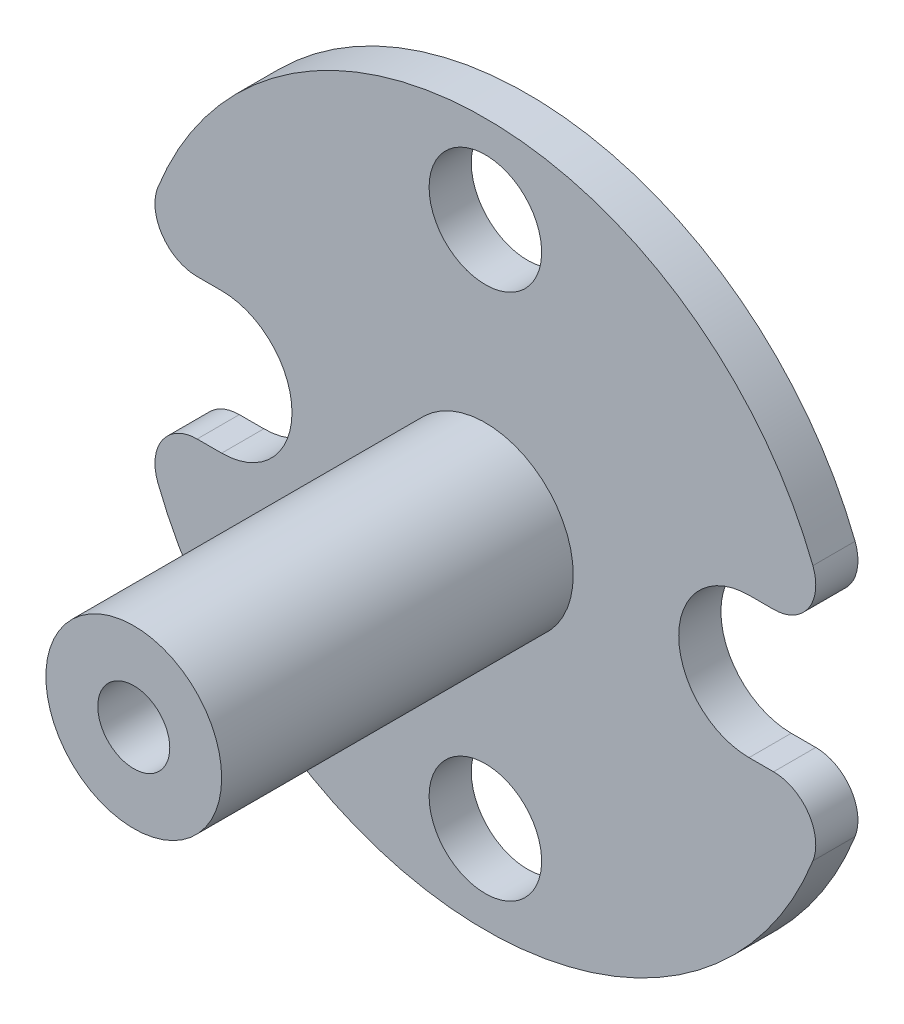
SolidWorks part; units mm, degrees
material "Plain Carbon Steel"
ref_plane "Front Plane" through (0, 0, 0) normal (0, 0, 1) x (1, 0, 0)
ref_plane "Top Plane" through (0, 0, 0) normal (0, 1, 0) x (1, 0, 0)
ref_plane "Right Plane" through (0, 0, 0) normal (1, 0, 0) x (0, 0, -1)
sketch "Plate Profile Sketch" plane through (0, 0, 0) normal (0, 0, 1) x (1, 0, 0)
  line L0 (-19.05, 5.08) -> (-24.8868, 5.08)
  line L1 (-19.05, -5.08) -> (-24.8868, -5.08)
  line L3 (19.05, -5.08) -> (24.8868, -5.08)
  line L4 (19.05, 5.08) -> (24.8868, 5.08)
  arc A0 (-24.8868, -5.08) -> (24.8868, -5.08) centre (0, 0) ccw
  circle A1 centre (0, 0) radius 19.05 construction
  arc A2 (-19.05, -5.08) -> (-19.05, 5.08) centre (-19.05, 0) ccw
  arc A3 (19.05, -5.08) -> (19.05, 5.08) centre (19.05, 0) cw
  arc A4 (24.8868, 5.08) -> (-24.8868, 5.08) centre (0, 0) ccw
  circle A5 centre (0, 19.05) radius 4.065
  circle A6 centre (0, -19.05) radius 4.065
  dimension "D1" = 50.8
  dimension "D2" = 38.1
  dimension "D3" = 10.16
  dimension "D4" = 8.13
extrude "Base Plate 0.12in" add sketch "Plate Profile Sketch" along normal blind 3.048
fillet "Plate Edge Fillet R0.12" radius 3.048 4 edges at (24.8868, -5.08, 1.524) (24.8868, 5.08, 1.524) (-24.8868, 5.08, 1.524) (-24.8868, -5.08, 1.524)
sketch "Hub Sketch Ø0.5" plane through (0, 0, 3.048) normal (0, 0, 1) x (1, 0, 0)
  circle A0 centre (0, 0) radius 6.35
  dimension "D1" = 12.7
extrude "Hub Ø0.5 x 1in" add sketch "Hub Sketch Ø0.5" along normal blind 25.4
sketch "Tapped Hole Position Sketch" plane through (0, 0, 28.448) normal (0, 0, 1) x (1, 0, 0)
  point P0 (0, 0)
hole_wizard "Hub Tapped Hole #10-24" positions "3DSketch1" profile "Sketch5" tap size "#10-24" standard "ANSI Inch"
sketch3d "3DSketch1"
  point P0 (0, 0, 0)
  point P3 (0, 0, 28.448)
sketch "Sketch5" plane through (0, 0, 28.448) normal (1, 0, 0) x (0, -1, 0)
  line L0 (0, 0) -> (0, 26.4721)
  line L1 (0, 26.4721) -> (2.45, 25)
  line L2 (2.45, 25) -> (2.45, 23)
  line L3 (2.45, 23) -> (2.6, 23)
  line L4 (2.6, 23) -> (2.6, 0)
  line L5 (2.6, 0) -> (0, 0)
  line L10 (0, 26.4721) -> (-2.45, 25) construction
  line L11 (0, -6.35) -> (0, 107.95) construction
  dimension "Tap Drill Dia." = 4.9
  dimension "Tap Drill Depth" = 25
  dimension "Thread Major Dia." = 5.2
  dimension "Thread Depth" = 23
  dimension "Drill Angle" = 118
